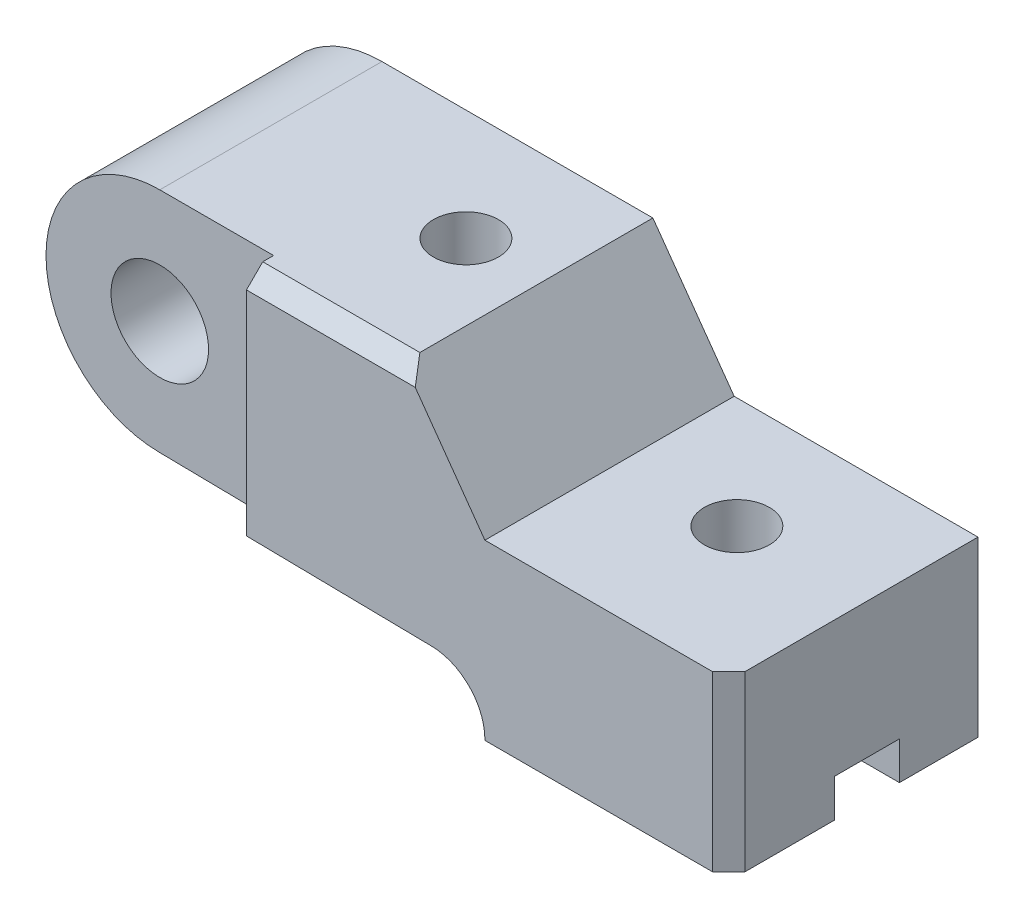
ISO-10303-21;
HEADER;
FILE_DESCRIPTION(('STEP AP214'),'2;1');
FILE_NAME('part.step','',(''),(''),'','','');
FILE_SCHEMA(('AUTOMOTIVE_DESIGN { 1 0 10303 214 1 1 1 1 }'));
ENDSEC;
DATA;
#1=APPLICATION_CONTEXT('core data for automotive mechanical design processes');
#2=APPLICATION_PROTOCOL_DEFINITION('international standard','automotive_design',2000,#1);
#3=PRODUCT_CONTEXT('',#1,'mechanical');
#4=PRODUCT('Part','Part','',(#3));
#5=PRODUCT_RELATED_PRODUCT_CATEGORY('part','',(#4));
#6=PRODUCT_DEFINITION_FORMATION('','',#4);
#7=PRODUCT_DEFINITION_CONTEXT('part definition',#1,'design');
#8=PRODUCT_DEFINITION('design','',#6,#7);
#9=PRODUCT_DEFINITION_SHAPE('','',#8);
#10=(LENGTH_UNIT() NAMED_UNIT(*) SI_UNIT(.MILLI.,.METRE.));
#11=(NAMED_UNIT(*) PLANE_ANGLE_UNIT() SI_UNIT($,.RADIAN.));
#12=(NAMED_UNIT(*) SI_UNIT($,.STERADIAN.) SOLID_ANGLE_UNIT());
#13=UNCERTAINTY_MEASURE_WITH_UNIT(LENGTH_MEASURE(1.E-05),#10,'distance_accuracy_value','');
#14=(GEOMETRIC_REPRESENTATION_CONTEXT(3) GLOBAL_UNCERTAINTY_ASSIGNED_CONTEXT((#13)) GLOBAL_UNIT_ASSIGNED_CONTEXT((#10,
#11,#12)) REPRESENTATION_CONTEXT('',''));
#15=CARTESIAN_POINT('',(0.,0.,0.));
#16=DIRECTION('',(0.,0.,1.));
#17=DIRECTION('',(1.,0.,0.));
#18=AXIS2_PLACEMENT_3D('',#15,#16,#17);
#19=CARTESIAN_POINT('',(0.,-25.,26.5));
#20=DIRECTION('',(0.,1.,0.));
#21=DIRECTION('',(0.,0.,1.));
#22=AXIS2_PLACEMENT_3D('',#19,#20,#21);
#23=PLANE('',#22);
#24=DIRECTION('',(1.,0.,0.));
#25=VECTOR('',#24,1.);
#26=CARTESIAN_POINT('',(0.,-25.,26.5));
#27=LINE('',#26,#25);
#28=CARTESIAN_POINT('',(21.,-25.,26.5));
#29=VERTEX_POINT('',#28);
#30=CARTESIAN_POINT('',(45.,-25.,26.5));
#31=VERTEX_POINT('',#30);
#32=EDGE_CURVE('E339',#29,#31,#27,.T.);
#33=ORIENTED_EDGE('',*,*,#32,.F.);
#34=CARTESIAN_POINT('',(21.,-25.,20.5));
#35=DIRECTION('',(0.,1.,0.));
#36=DIRECTION('',(0.,0.,1.));
#37=AXIS2_PLACEMENT_3D('',#34,#35,#36);
#38=CIRCLE('',#37,6.);
#39=CARTESIAN_POINT('',(21.,-25.,14.5));
#40=VERTEX_POINT('',#39);
#41=EDGE_CURVE('E223',#29,#40,#38,.T.);
#42=ORIENTED_EDGE('',*,*,#41,.T.);
#43=DIRECTION('',(1.,0.,0.));
#44=VECTOR('',#43,1.);
#45=CARTESIAN_POINT('',(0.,-25.,14.5));
#46=LINE('',#45,#44);
#47=CARTESIAN_POINT('',(45.,-25.,14.5));
#48=VERTEX_POINT('',#47);
#49=EDGE_CURVE('E338',#40,#48,#46,.T.);
#50=ORIENTED_EDGE('',*,*,#49,.T.);
#51=DIRECTION('',(0.,0.,1.));
#52=VECTOR('',#51,1.);
#53=CARTESIAN_POINT('',(45.,-25.,26.5));
#54=LINE('',#53,#52);
#55=EDGE_CURVE('E684',#48,#31,#54,.T.);
#56=ORIENTED_EDGE('',*,*,#55,.T.);
#57=EDGE_LOOP('',(#33,#42,#50,#56));
#58=FACE_BOUND('',#57,.T.);
#59=ADVANCED_FACE('F43',(#58),#23,.F.);
#60=CARTESIAN_POINT('',(0.,0.,41.));
#61=DIRECTION('',(1.,0.,0.));
#62=DIRECTION('',(0.,0.,-1.));
#63=AXIS2_PLACEMENT_3D('',#60,#61,#62);
#64=PLANE('',#63);
#65=DIRECTION('',(0.,0.,1.));
#66=VECTOR('',#65,1.);
#67=CARTESIAN_POINT('',(0.,-31.6923440991361,0.));
#68=LINE('',#67,#66);
#69=CARTESIAN_POINT('',(0.,-31.6923440991361,0.));
#70=VERTEX_POINT('',#69);
#71=CARTESIAN_POINT('',(0.,-31.6923440991361,14.5));
#72=VERTEX_POINT('',#71);
#73=EDGE_CURVE('E259',#70,#72,#68,.T.);
#74=ORIENTED_EDGE('',*,*,#73,.F.);
#75=DIRECTION('',(0.,-1.,0.));
#76=VECTOR('',#75,1.);
#77=CARTESIAN_POINT('',(0.,0.,0.));
#78=LINE('',#77,#76);
#79=CARTESIAN_POINT('',(0.,-32.,0.));
#80=VERTEX_POINT('',#79);
#81=EDGE_CURVE('E353',#70,#80,#78,.T.);
#82=ORIENTED_EDGE('',*,*,#81,.T.);
#83=DIRECTION('',(0.,0.,-1.));
#84=VECTOR('',#83,1.);
#85=CARTESIAN_POINT('',(0.,-32.,41.));
#86=LINE('',#85,#84);
#87=CARTESIAN_POINT('',(0.,-32.,14.5));
#88=VERTEX_POINT('',#87);
#89=EDGE_CURVE('E270',#88,#80,#86,.T.);
#90=ORIENTED_EDGE('',*,*,#89,.F.);
#91=DIRECTION('',(0.,1.,0.));
#92=VECTOR('',#91,1.);
#93=CARTESIAN_POINT('',(0.,-25.,14.5));
#94=LINE('',#93,#92);
#95=EDGE_CURVE('E677',#88,#72,#94,.T.);
#96=ORIENTED_EDGE('',*,*,#95,.T.);
#97=EDGE_LOOP('',(#74,#82,#90,#96));
#98=FACE_BOUND('',#97,.T.);
#99=ADVANCED_FACE('F276',(#98),#64,.F.);
#100=CARTESIAN_POINT('',(0.,-31.6923440991361,26.5));
#101=VERTEX_POINT('',#100);
#102=CARTESIAN_POINT('',(0.,-31.6923440991361,41.));
#103=VERTEX_POINT('',#102);
#104=EDGE_CURVE('E262',#101,#103,#68,.T.);
#105=ORIENTED_EDGE('',*,*,#104,.F.);
#106=DIRECTION('',(0.,-1.,0.));
#107=VECTOR('',#106,1.);
#108=CARTESIAN_POINT('',(0.,-32.,26.5));
#109=LINE('',#108,#107);
#110=CARTESIAN_POINT('',(0.,-32.,26.5));
#111=VERTEX_POINT('',#110);
#112=EDGE_CURVE('E685',#101,#111,#109,.T.);
#113=ORIENTED_EDGE('',*,*,#112,.T.);
#114=CARTESIAN_POINT('',(0.,-32.,41.));
#115=VERTEX_POINT('',#114);
#116=EDGE_CURVE('E267',#115,#111,#86,.T.);
#117=ORIENTED_EDGE('',*,*,#116,.F.);
#118=CARTESIAN_POINT('',(-9.99881677808259,-31.846172049568,41.));
#119=DIRECTION('',(0.,0.,-1.));
#120=DIRECTION('',(0.999881677808259,0.0153827950431833,0.));
#121=AXIS2_PLACEMENT_3D('',#118,#119,#120);
#122=CIRCLE('',#121,10.);
#123=EDGE_CURVE('E204',#103,#115,#122,.T.);
#124=ORIENTED_EDGE('',*,*,#123,.F.);
#125=EDGE_LOOP('',(#105,#113,#117,#124));
#126=FACE_BOUND('',#125,.T.);
#127=ADVANCED_FACE('F287',(#126),#64,.F.);
#128=CARTESIAN_POINT('',(45.,-32.,41.));
#129=DIRECTION('',(0.,1.,0.));
#130=DIRECTION('',(0.,0.,1.));
#131=AXIS2_PLACEMENT_3D('',#128,#129,#130);
#132=PLANE('',#131);
#133=DIRECTION('',(0.,0.,-1.));
#134=VECTOR('',#133,1.);
#135=CARTESIAN_POINT('',(45.,-32.,41.));
#136=LINE('',#135,#134);
#137=CARTESIAN_POINT('',(45.,-32.,43.));
#138=VERTEX_POINT('',#137);
#139=CARTESIAN_POINT('',(45.,-32.,26.5));
#140=VERTEX_POINT('',#139);
#141=EDGE_CURVE('E366',#138,#140,#136,.T.);
#142=ORIENTED_EDGE('',*,*,#141,.F.);
#143=DIRECTION('',(-0.707106781186546,0.,0.707106781186549));
#144=VECTOR('',#143,1.);
#145=CARTESIAN_POINT('',(42.,-32.,46.));
#146=LINE('',#145,#144);
#147=CARTESIAN_POINT('',(42.,-32.,46.));
#148=VERTEX_POINT('',#147);
#149=EDGE_CURVE('E11',#138,#148,#146,.T.);
#150=ORIENTED_EDGE('',*,*,#149,.T.);
#151=DIRECTION('',(1.,0.,0.));
#152=VECTOR('',#151,1.);
#153=CARTESIAN_POINT('',(0.,-32.,46.));
#154=LINE('',#153,#152);
#155=CARTESIAN_POINT('',(0.,-32.,46.));
#156=VERTEX_POINT('',#155);
#157=EDGE_CURVE('E176',#156,#148,#154,.T.);
#158=ORIENTED_EDGE('',*,*,#157,.F.);
#159=DIRECTION('',(0.,0.,-1.));
#160=VECTOR('',#159,1.);
#161=CARTESIAN_POINT('',(0.,-32.,46.));
#162=LINE('',#161,#160);
#163=EDGE_CURVE('E181',#156,#115,#162,.T.);
#164=ORIENTED_EDGE('',*,*,#163,.T.);
#165=ORIENTED_EDGE('',*,*,#116,.T.);
#166=DIRECTION('',(1.,0.,0.));
#167=VECTOR('',#166,1.);
#168=CARTESIAN_POINT('',(0.,-32.,26.5));
#169=LINE('',#168,#167);
#170=EDGE_CURVE('E350',#111,#140,#169,.T.);
#171=ORIENTED_EDGE('',*,*,#170,.T.);
#172=EDGE_LOOP('',(#142,#150,#158,#164,#165,#171));
#173=FACE_BOUND('',#172,.T.);
#174=ADVANCED_FACE('F178',(#173),#132,.F.);
#175=CARTESIAN_POINT('',(45.,-32.,14.5));
#176=VERTEX_POINT('',#175);
#177=CARTESIAN_POINT('',(45.,-32.,0.));
#178=VERTEX_POINT('',#177);
#179=EDGE_CURVE('E362',#176,#178,#136,.T.);
#180=ORIENTED_EDGE('',*,*,#179,.F.);
#181=DIRECTION('',(1.,0.,0.));
#182=VECTOR('',#181,1.);
#183=CARTESIAN_POINT('',(0.,-32.,14.5));
#184=LINE('',#183,#182);
#185=EDGE_CURVE('E341',#88,#176,#184,.T.);
#186=ORIENTED_EDGE('',*,*,#185,.F.);
#187=ORIENTED_EDGE('',*,*,#89,.T.);
#188=DIRECTION('',(1.,0.,0.));
#189=VECTOR('',#188,1.);
#190=CARTESIAN_POINT('',(45.,-32.,0.));
#191=LINE('',#190,#189);
#192=EDGE_CURVE('E352',#80,#178,#191,.T.);
#193=ORIENTED_EDGE('',*,*,#192,.T.);
#194=EDGE_LOOP('',(#180,#186,#187,#193));
#195=FACE_BOUND('',#194,.T.);
#196=ADVANCED_FACE('F286',(#195),#132,.F.);
#197=CARTESIAN_POINT('',(45.,0.,41.));
#198=DIRECTION('',(-1.,0.,0.));
#199=DIRECTION('',(0.,0.,1.));
#200=AXIS2_PLACEMENT_3D('',#197,#198,#199);
#201=PLANE('',#200);
#202=DIRECTION('',(0.,0.,-1.));
#203=VECTOR('',#202,1.);
#204=CARTESIAN_POINT('',(45.,0.,41.));
#205=LINE('',#204,#203);
#206=CARTESIAN_POINT('',(45.,0.,43.));
#207=VERTEX_POINT('',#206);
#208=CARTESIAN_POINT('',(45.,0.,0.));
#209=VERTEX_POINT('',#208);
#210=EDGE_CURVE('E364',#207,#209,#205,.T.);
#211=ORIENTED_EDGE('',*,*,#210,.F.);
#212=DIRECTION('',(0.,-1.,0.));
#213=VECTOR('',#212,1.);
#214=CARTESIAN_POINT('',(45.,-32.,43.));
#215=LINE('',#214,#213);
#216=EDGE_CURVE('E55',#207,#138,#215,.T.);
#217=ORIENTED_EDGE('',*,*,#216,.T.);
#218=ORIENTED_EDGE('',*,*,#141,.T.);
#219=DIRECTION('',(0.,-1.,0.));
#220=VECTOR('',#219,1.);
#221=CARTESIAN_POINT('',(45.,-32.,26.5));
#222=LINE('',#221,#220);
#223=EDGE_CURVE('E249',#31,#140,#222,.T.);
#224=ORIENTED_EDGE('',*,*,#223,.F.);
#225=ORIENTED_EDGE('',*,*,#55,.F.);
#226=DIRECTION('',(0.,1.,0.));
#227=VECTOR('',#226,1.);
#228=CARTESIAN_POINT('',(45.,-25.,14.5));
#229=LINE('',#228,#227);
#230=EDGE_CURVE('E380',#176,#48,#229,.T.);
#231=ORIENTED_EDGE('',*,*,#230,.F.);
#232=ORIENTED_EDGE('',*,*,#179,.T.);
#233=DIRECTION('',(0.,1.,0.));
#234=VECTOR('',#233,1.);
#235=CARTESIAN_POINT('',(45.,0.,0.));
#236=LINE('',#235,#234);
#237=EDGE_CURVE('E358',#178,#209,#236,.T.);
#238=ORIENTED_EDGE('',*,*,#237,.T.);
#239=EDGE_LOOP('',(#211,#217,#218,#224,#225,#231,#232,#238));
#240=FACE_BOUND('',#239,.T.);
#241=ADVANCED_FACE('F375',(#240),#201,.F.);
#242=CARTESIAN_POINT('',(0.,0.,41.));
#243=DIRECTION('',(0.,-1.,0.));
#244=DIRECTION('',(0.,0.,-1.));
#245=AXIS2_PLACEMENT_3D('',#242,#243,#244);
#246=PLANE('',#245);
#247=CARTESIAN_POINT('',(21.,0.,20.5));
#248=DIRECTION('',(0.,-1.,0.));
#249=DIRECTION('',(0.,0.,-1.));
#250=AXIS2_PLACEMENT_3D('',#247,#248,#249);
#251=CIRCLE('',#250,6.);
#252=CARTESIAN_POINT('',(21.,0.,14.5));
#253=VERTEX_POINT('',#252);
#254=EDGE_CURVE('E224',#253,#253,#251,.T.);
#255=ORIENTED_EDGE('',*,*,#254,.T.);
#256=EDGE_LOOP('',(#255));
#257=FACE_BOUND('',#256,.T.);
#258=DIRECTION('',(-1.,0.,0.));
#259=VECTOR('',#258,1.);
#260=CARTESIAN_POINT('',(0.,0.,46.));
#261=LINE('',#260,#259);
#262=CARTESIAN_POINT('',(42.,0.,46.));
#263=VERTEX_POINT('',#262);
#264=CARTESIAN_POINT('',(0.,0.,46.));
#265=VERTEX_POINT('',#264);
#266=EDGE_CURVE('E190',#263,#265,#261,.T.);
#267=ORIENTED_EDGE('',*,*,#266,.F.);
#268=DIRECTION('',(0.707106781186546,0.,-0.707106781186549));
#269=VECTOR('',#268,1.);
#270=CARTESIAN_POINT('',(42.,0.,46.));
#271=LINE('',#270,#269);
#272=EDGE_CURVE('E69',#263,#207,#271,.T.);
#273=ORIENTED_EDGE('',*,*,#272,.T.);
#274=ORIENTED_EDGE('',*,*,#210,.T.);
#275=DIRECTION('',(-1.,0.,0.));
#276=VECTOR('',#275,1.);
#277=CARTESIAN_POINT('',(0.,0.,0.));
#278=LINE('',#277,#276);
#279=CARTESIAN_POINT('',(0.,0.,0.));
#280=VERTEX_POINT('',#279);
#281=EDGE_CURVE('E360',#209,#280,#278,.T.);
#282=ORIENTED_EDGE('',*,*,#281,.T.);
#283=DIRECTION('',(0.,0.,-1.));
#284=VECTOR('',#283,1.);
#285=CARTESIAN_POINT('',(0.,0.,41.));
#286=LINE('',#285,#284);
#287=EDGE_CURVE('E363',#265,#280,#286,.T.);
#288=ORIENTED_EDGE('',*,*,#287,.F.);
#289=EDGE_LOOP('',(#267,#273,#274,#282,#288));
#290=FACE_BOUND('',#289,.T.);
#291=ADVANCED_FACE('F387',(#257,#290),#246,.F.);
#292=CARTESIAN_POINT('',(0.,0.,41.));
#293=DIRECTION('',(0.,0.,-1.));
#294=DIRECTION('',(-1.,0.,0.));
#295=AXIS2_PLACEMENT_3D('',#292,#293,#294);
#296=PLANE('',#295);
#297=CARTESIAN_POINT('',(-65.,8.11850586757146E-13,41.));
#298=DIRECTION('',(0.,0.,1.));
#299=DIRECTION('',(1.,0.,0.));
#300=AXIS2_PLACEMENT_3D('',#297,#298,#299);
#301=CIRCLE('',#300,9.);
#302=CARTESIAN_POINT('',(-56.,8.11850586757146E-13,41.));
#303=VERTEX_POINT('',#302);
#304=EDGE_CURVE('E401',#303,#303,#301,.T.);
#305=ORIENTED_EDGE('',*,*,#304,.F.);
#306=EDGE_LOOP('',(#305));
#307=FACE_BOUND('',#306,.T.);
#308=DIRECTION('',(0.999881677808259,-0.0153827950432186,0.));
#309=VECTOR('',#308,1.);
#310=CARTESIAN_POINT('',(-0.33838144817827,-21.9947941315666,41.));
#311=LINE('',#310,#309);
#312=CARTESIAN_POINT('',(-65.,-20.9999999999992,41.));
#313=VERTEX_POINT('',#312);
#314=CARTESIAN_POINT('',(-44.,-21.3230769230764,41.));
#315=VERTEX_POINT('',#314);
#316=EDGE_CURVE('E230',#313,#315,#311,.T.);
#317=ORIENTED_EDGE('',*,*,#316,.T.);
#318=DIRECTION('',(0.,1.,0.));
#319=VECTOR('',#318,1.);
#320=CARTESIAN_POINT('',(-44.,0.,41.));
#321=LINE('',#320,#319);
#322=CARTESIAN_POINT('',(-44.,21.0000000000008,41.));
#323=VERTEX_POINT('',#322);
#324=EDGE_CURVE('E200',#315,#323,#321,.T.);
#325=ORIENTED_EDGE('',*,*,#324,.T.);
#326=DIRECTION('',(1.,0.,0.));
#327=VECTOR('',#326,1.);
#328=CARTESIAN_POINT('',(0.,21.0000000000008,41.));
#329=LINE('',#328,#327);
#330=CARTESIAN_POINT('',(-65.,21.0000000000008,41.));
#331=VERTEX_POINT('',#330);
#332=EDGE_CURVE('E221',#331,#323,#329,.T.);
#333=ORIENTED_EDGE('',*,*,#332,.F.);
#334=CARTESIAN_POINT('',(-65.,8.11850586757146E-13,41.));
#335=DIRECTION('',(0.,0.,1.));
#336=DIRECTION('',(1.,0.,0.));
#337=AXIS2_PLACEMENT_3D('',#334,#335,#336);
#338=CIRCLE('',#337,21.);
#339=EDGE_CURVE('E243',#331,#313,#338,.T.);
#340=ORIENTED_EDGE('',*,*,#339,.T.);
#341=EDGE_LOOP('',(#317,#325,#333,#340));
#342=FACE_BOUND('',#341,.T.);
#343=ADVANCED_FACE('F582',(#307,#342),#296,.F.);
#344=CARTESIAN_POINT('',(0.,0.,0.));
#345=DIRECTION('',(0.,0.,-1.));
#346=DIRECTION('',(-1.,0.,0.));
#347=AXIS2_PLACEMENT_3D('',#344,#345,#346);
#348=PLANE('',#347);
#349=CARTESIAN_POINT('',(-65.,8.11850586757146E-13,0.));
#350=DIRECTION('',(0.,0.,-1.));
#351=DIRECTION('',(-1.,0.,0.));
#352=AXIS2_PLACEMENT_3D('',#349,#350,#351);
#353=CIRCLE('',#352,9.);
#354=CARTESIAN_POINT('',(-74.,8.11850586757146E-13,0.));
#355=VERTEX_POINT('',#354);
#356=EDGE_CURVE('E402',#355,#355,#353,.T.);
#357=ORIENTED_EDGE('',*,*,#356,.F.);
#358=EDGE_LOOP('',(#357));
#359=FACE_BOUND('',#358,.T.);
#360=ORIENTED_EDGE('',*,*,#81,.F.);
#361=CARTESIAN_POINT('',(-9.99881677808259,-31.846172049568,0.));
#362=DIRECTION('',(0.,0.,1.));
#363=DIRECTION('',(1.,0.,0.));
#364=AXIS2_PLACEMENT_3D('',#361,#362,#363);
#365=CIRCLE('',#364,10.);
#366=CARTESIAN_POINT('',(-9.9988167780826,-21.846172049568,0.));
#367=VERTEX_POINT('',#366);
#368=EDGE_CURVE('E228',#70,#367,#365,.T.);
#369=ORIENTED_EDGE('',*,*,#368,.T.);
#370=DIRECTION('',(0.999881677808259,-0.0153827950432186,0.));
#371=VECTOR('',#370,1.);
#372=CARTESIAN_POINT('',(-0.33838144817827,-21.9947941315666,0.));
#373=LINE('',#372,#371);
#374=CARTESIAN_POINT('',(-65.,-20.9999999999992,0.));
#375=VERTEX_POINT('',#374);
#376=EDGE_CURVE('E240',#375,#367,#373,.T.);
#377=ORIENTED_EDGE('',*,*,#376,.F.);
#378=CARTESIAN_POINT('',(-65.,8.11850586757146E-13,0.));
#379=DIRECTION('',(0.,0.,1.));
#380=DIRECTION('',(1.,0.,0.));
#381=AXIS2_PLACEMENT_3D('',#378,#379,#380);
#382=CIRCLE('',#381,21.);
#383=CARTESIAN_POINT('',(-65.,21.0000000000008,0.));
#384=VERTEX_POINT('',#383);
#385=EDGE_CURVE('E234',#384,#375,#382,.T.);
#386=ORIENTED_EDGE('',*,*,#385,.F.);
#387=DIRECTION('',(1.,0.,0.));
#388=VECTOR('',#387,1.);
#389=CARTESIAN_POINT('',(0.,21.0000000000008,0.));
#390=LINE('',#389,#388);
#391=CARTESIAN_POINT('',(-15.,21.0000000000008,0.));
#392=VERTEX_POINT('',#391);
#393=EDGE_CURVE('E235',#384,#392,#390,.T.);
#394=ORIENTED_EDGE('',*,*,#393,.T.);
#395=DIRECTION('',(0.581238193719081,-0.813733471206746,0.));
#396=VECTOR('',#395,1.);
#397=CARTESIAN_POINT('',(0.,0.,0.));
#398=LINE('',#397,#396);
#399=EDGE_CURVE('E226',#392,#280,#398,.T.);
#400=ORIENTED_EDGE('',*,*,#399,.T.);
#401=ORIENTED_EDGE('',*,*,#281,.F.);
#402=ORIENTED_EDGE('',*,*,#237,.F.);
#403=ORIENTED_EDGE('',*,*,#192,.F.);
#404=EDGE_LOOP('',(#360,#369,#377,#386,#394,#400,#401,#402,#403));
#405=FACE_BOUND('',#404,.T.);
#406=ADVANCED_FACE('F328',(#359,#405),#348,.T.);
#407=CARTESIAN_POINT('',(0.,-32.,26.5));
#408=DIRECTION('',(0.,0.,1.));
#409=DIRECTION('',(1.,0.,0.));
#410=AXIS2_PLACEMENT_3D('',#407,#408,#409);
#411=PLANE('',#410);
#412=CARTESIAN_POINT('',(0.,-25.,26.5));
#413=VERTEX_POINT('',#412);
#414=EDGE_CURVE('E345',#413,#29,#27,.T.);
#415=ORIENTED_EDGE('',*,*,#414,.T.);
#416=ORIENTED_EDGE('',*,*,#32,.T.);
#417=ORIENTED_EDGE('',*,*,#223,.T.);
#418=ORIENTED_EDGE('',*,*,#170,.F.);
#419=ORIENTED_EDGE('',*,*,#112,.F.);
#420=EDGE_CURVE('E261',#413,#101,#109,.T.);
#421=ORIENTED_EDGE('',*,*,#420,.F.);
#422=EDGE_LOOP('',(#415,#416,#417,#418,#419,#421));
#423=FACE_BOUND('',#422,.T.);
#424=ADVANCED_FACE('F325',(#423),#411,.F.);
#425=CARTESIAN_POINT('',(0.,-25.,14.5));
#426=VERTEX_POINT('',#425);
#427=EDGE_CURVE('E335',#426,#40,#46,.T.);
#428=ORIENTED_EDGE('',*,*,#427,.T.);
#429=EDGE_CURVE('E220',#40,#29,#38,.T.);
#430=ORIENTED_EDGE('',*,*,#429,.T.);
#431=ORIENTED_EDGE('',*,*,#414,.F.);
#432=DIRECTION('',(0.,0.,1.));
#433=VECTOR('',#432,1.);
#434=CARTESIAN_POINT('',(0.,-25.,26.5));
#435=LINE('',#434,#433);
#436=EDGE_CURVE('E337',#426,#413,#435,.T.);
#437=ORIENTED_EDGE('',*,*,#436,.F.);
#438=EDGE_LOOP('',(#428,#430,#431,#437));
#439=FACE_BOUND('',#438,.T.);
#440=ADVANCED_FACE('F315',(#439),#23,.F.);
#441=CARTESIAN_POINT('',(0.,-25.,14.5));
#442=DIRECTION('',(0.,0.,-1.));
#443=DIRECTION('',(-1.,0.,0.));
#444=AXIS2_PLACEMENT_3D('',#441,#442,#443);
#445=PLANE('',#444);
#446=ORIENTED_EDGE('',*,*,#49,.F.);
#447=ORIENTED_EDGE('',*,*,#427,.F.);
#448=EDGE_CURVE('E680',#72,#426,#94,.T.);
#449=ORIENTED_EDGE('',*,*,#448,.F.);
#450=ORIENTED_EDGE('',*,*,#95,.F.);
#451=ORIENTED_EDGE('',*,*,#185,.T.);
#452=ORIENTED_EDGE('',*,*,#230,.T.);
#453=EDGE_LOOP('',(#446,#447,#449,#450,#451,#452));
#454=FACE_BOUND('',#453,.T.);
#455=ADVANCED_FACE('F322',(#454),#445,.F.);
#456=CARTESIAN_POINT('',(0.,0.,0.));
#457=DIRECTION('',(-1.,0.,0.));
#458=DIRECTION('',(0.,0.,1.));
#459=AXIS2_PLACEMENT_3D('',#456,#457,#458);
#460=PLANE('',#459);
#461=ORIENTED_EDGE('',*,*,#436,.T.);
#462=ORIENTED_EDGE('',*,*,#420,.T.);
#463=EDGE_CURVE('E239',#72,#101,#68,.T.);
#464=ORIENTED_EDGE('',*,*,#463,.F.);
#465=ORIENTED_EDGE('',*,*,#448,.T.);
#466=EDGE_LOOP('',(#461,#462,#464,#465));
#467=FACE_BOUND('',#466,.T.);
#468=ADVANCED_FACE('F326',(#467),#460,.F.);
#469=CARTESIAN_POINT('',(-9.99881677808259,-31.846172049568,0.));
#470=DIRECTION('',(0.,0.,1.));
#471=DIRECTION('',(1.,0.,0.));
#472=AXIS2_PLACEMENT_3D('',#469,#470,#471);
#473=CYLINDRICAL_SURFACE('',#472,10.);
#474=ORIENTED_EDGE('',*,*,#104,.T.);
#475=ORIENTED_EDGE('',*,*,#123,.T.);
#476=ORIENTED_EDGE('',*,*,#163,.F.);
#477=CARTESIAN_POINT('',(-9.99881677808259,-31.846172049568,46.));
#478=DIRECTION('',(0.,0.,1.));
#479=DIRECTION('',(1.,0.,0.));
#480=AXIS2_PLACEMENT_3D('',#477,#478,#479);
#481=CIRCLE('',#480,10.);
#482=CARTESIAN_POINT('',(-9.9988167780826,-21.846172049568,46.));
#483=VERTEX_POINT('',#482);
#484=EDGE_CURVE('E189',#483,#156,#481,.F.);
#485=ORIENTED_EDGE('',*,*,#484,.F.);
#486=DIRECTION('',(0.,0.,1.));
#487=VECTOR('',#486,1.);
#488=CARTESIAN_POINT('',(-9.9988167780826,-21.846172049568,0.));
#489=LINE('',#488,#487);
#490=EDGE_CURVE('E247',#367,#483,#489,.T.);
#491=ORIENTED_EDGE('',*,*,#490,.F.);
#492=ORIENTED_EDGE('',*,*,#368,.F.);
#493=ORIENTED_EDGE('',*,*,#73,.T.);
#494=ORIENTED_EDGE('',*,*,#463,.T.);
#495=EDGE_LOOP('',(#474,#475,#476,#485,#491,#492,#493,#494));
#496=FACE_BOUND('',#495,.T.);
#497=ADVANCED_FACE('F203',(#496),#473,.F.);
#498=CARTESIAN_POINT('',(-0.33838144817827,-21.9947941315666,0.));
#499=DIRECTION('',(-0.0153827950432186,-0.999881677808259,0.));
#500=DIRECTION('',(0.999881677808259,-0.0153827950432186,0.));
#501=AXIS2_PLACEMENT_3D('',#498,#499,#500);
#502=PLANE('',#501);
#503=CARTESIAN_POINT('',(-29.,-21.5538461538459,20.5));
#504=DIRECTION('',(-0.0153827950432186,-0.999881677808259,0.));
#505=DIRECTION('',(-0.999881677808259,0.0153827950432186,0.));
#506=AXIS2_PLACEMENT_3D('',#503,#504,#505);
#507=ELLIPSE('',#506,6.00071001716124,6.);
#508=CARTESIAN_POINT('',(-35.,-21.4615384615381,20.5));
#509=VERTEX_POINT('',#508);
#510=EDGE_CURVE('E206',#509,#509,#507,.T.);
#511=ORIENTED_EDGE('',*,*,#510,.F.);
#512=EDGE_LOOP('',(#511));
#513=FACE_BOUND('',#512,.T.);
#514=ORIENTED_EDGE('',*,*,#316,.F.);
#515=DIRECTION('',(0.,0.,1.));
#516=VECTOR('',#515,1.);
#517=CARTESIAN_POINT('',(-65.,-20.9999999999992,0.));
#518=LINE('',#517,#516);
#519=EDGE_CURVE('E252',#375,#313,#518,.T.);
#520=ORIENTED_EDGE('',*,*,#519,.F.);
#521=ORIENTED_EDGE('',*,*,#376,.T.);
#522=ORIENTED_EDGE('',*,*,#490,.T.);
#523=DIRECTION('',(0.999881677808259,-0.0153827950432186,0.));
#524=VECTOR('',#523,1.);
#525=CARTESIAN_POINT('',(-0.33838144817827,-21.9947941315666,46.));
#526=LINE('',#525,#524);
#527=CARTESIAN_POINT('',(-44.,-21.3230769230764,46.));
#528=VERTEX_POINT('',#527);
#529=EDGE_CURVE('E193',#528,#483,#526,.T.);
#530=ORIENTED_EDGE('',*,*,#529,.F.);
#531=DIRECTION('',(0.,0.,-1.));
#532=VECTOR('',#531,1.);
#533=CARTESIAN_POINT('',(-44.,-21.3230769230764,46.));
#534=LINE('',#533,#532);
#535=EDGE_CURVE('E208',#528,#315,#534,.T.);
#536=ORIENTED_EDGE('',*,*,#535,.T.);
#537=EDGE_LOOP('',(#514,#520,#521,#522,#530,#536));
#538=FACE_BOUND('',#537,.T.);
#539=ADVANCED_FACE('F413',(#513,#538),#502,.T.);
#540=CARTESIAN_POINT('',(-65.,8.11850586757146E-13,0.));
#541=DIRECTION('',(0.,0.,1.));
#542=DIRECTION('',(1.,0.,0.));
#543=AXIS2_PLACEMENT_3D('',#540,#541,#542);
#544=CYLINDRICAL_SURFACE('',#543,21.);
#545=ORIENTED_EDGE('',*,*,#339,.F.);
#546=DIRECTION('',(0.,0.,1.));
#547=VECTOR('',#546,1.);
#548=CARTESIAN_POINT('',(-65.,21.0000000000008,0.));
#549=LINE('',#548,#547);
#550=EDGE_CURVE('E254',#384,#331,#549,.T.);
#551=ORIENTED_EDGE('',*,*,#550,.F.);
#552=ORIENTED_EDGE('',*,*,#385,.T.);
#553=ORIENTED_EDGE('',*,*,#519,.T.);
#554=EDGE_LOOP('',(#545,#551,#552,#553));
#555=FACE_BOUND('',#554,.T.);
#556=ADVANCED_FACE('F428',(#555),#544,.T.);
#557=CARTESIAN_POINT('',(0.,21.0000000000008,0.));
#558=DIRECTION('',(0.,-1.,0.));
#559=DIRECTION('',(0.,0.,-1.));
#560=AXIS2_PLACEMENT_3D('',#557,#558,#559);
#561=PLANE('',#560);
#562=CARTESIAN_POINT('',(-29.,21.0000000000008,20.5));
#563=DIRECTION('',(0.,1.,0.));
#564=DIRECTION('',(0.,0.,1.));
#565=AXIS2_PLACEMENT_3D('',#562,#563,#564);
#566=CIRCLE('',#565,6.);
#567=CARTESIAN_POINT('',(-29.,21.0000000000008,26.5));
#568=VERTEX_POINT('',#567);
#569=EDGE_CURVE('E205',#568,#568,#566,.T.);
#570=ORIENTED_EDGE('',*,*,#569,.F.);
#571=EDGE_LOOP('',(#570));
#572=FACE_BOUND('',#571,.T.);
#573=DIRECTION('',(0.,0.,-1.));
#574=VECTOR('',#573,1.);
#575=CARTESIAN_POINT('',(-44.,21.0000000000008,46.));
#576=LINE('',#575,#574);
#577=CARTESIAN_POINT('',(-44.,21.0000000000008,43.));
#578=VERTEX_POINT('',#577);
#579=EDGE_CURVE('E201',#578,#323,#576,.T.);
#580=ORIENTED_EDGE('',*,*,#579,.F.);
#581=DIRECTION('',(1.,0.,0.));
#582=VECTOR('',#581,1.);
#583=CARTESIAN_POINT('',(-15.,21.0000000000008,43.));
#584=LINE('',#583,#582);
#585=CARTESIAN_POINT('',(-15.,21.0000000000008,43.));
#586=VERTEX_POINT('',#585);
#587=EDGE_CURVE('E393',#578,#586,#584,.T.);
#588=ORIENTED_EDGE('',*,*,#587,.T.);
#589=DIRECTION('',(0.,0.,1.));
#590=VECTOR('',#589,1.);
#591=CARTESIAN_POINT('',(-15.,21.0000000000008,0.));
#592=LINE('',#591,#590);
#593=EDGE_CURVE('E253',#392,#586,#592,.T.);
#594=ORIENTED_EDGE('',*,*,#593,.F.);
#595=ORIENTED_EDGE('',*,*,#393,.F.);
#596=ORIENTED_EDGE('',*,*,#550,.T.);
#597=ORIENTED_EDGE('',*,*,#332,.T.);
#598=EDGE_LOOP('',(#580,#588,#594,#595,#596,#597));
#599=FACE_BOUND('',#598,.T.);
#600=ADVANCED_FACE('F422',(#572,#599),#561,.F.);
#601=CARTESIAN_POINT('',(0.,0.,0.));
#602=DIRECTION('',(-0.813733471206746,-0.581238193719081,0.));
#603=DIRECTION('',(0.581238193719081,-0.813733471206746,0.));
#604=AXIS2_PLACEMENT_3D('',#601,#602,#603);
#605=PLANE('',#604);
#606=ORIENTED_EDGE('',*,*,#593,.T.);
#607=DIRECTION('',(0.450834817333701,-0.631168744267206,0.631168744267209));
#608=VECTOR('',#607,1.);
#609=CARTESIAN_POINT('',(-10.2439024390246,14.341463414635,49.6585365853658));
#610=LINE('',#609,#608);
#611=CARTESIAN_POINT('',(-12.8571428571429,18.0000000000008,46.));
#612=VERTEX_POINT('',#611);
#613=EDGE_CURVE('E391',#586,#612,#610,.T.);
#614=ORIENTED_EDGE('',*,*,#613,.T.);
#615=DIRECTION('',(-0.581238193719081,0.813733471206746,0.));
#616=VECTOR('',#615,1.);
#617=CARTESIAN_POINT('',(0.,0.,46.));
#618=LINE('',#617,#616);
#619=EDGE_CURVE('E665',#265,#612,#618,.T.);
#620=ORIENTED_EDGE('',*,*,#619,.F.);
#621=ORIENTED_EDGE('',*,*,#287,.T.);
#622=ORIENTED_EDGE('',*,*,#399,.F.);
#623=EDGE_LOOP('',(#606,#614,#620,#621,#622));
#624=FACE_BOUND('',#623,.T.);
#625=ADVANCED_FACE('F417',(#624),#605,.F.);
#626=CARTESIAN_POINT('',(-29.,-28.9999999999992,20.5));
#627=DIRECTION('',(0.,1.,0.));
#628=DIRECTION('',(0.,0.,1.));
#629=AXIS2_PLACEMENT_3D('',#626,#627,#628);
#630=CYLINDRICAL_SURFACE('',#629,6.);
#631=ORIENTED_EDGE('',*,*,#510,.T.);
#632=EDGE_LOOP('',(#631));
#633=FACE_BOUND('',#632,.T.);
#634=ORIENTED_EDGE('',*,*,#569,.T.);
#635=EDGE_LOOP('',(#634));
#636=FACE_BOUND('',#635,.T.);
#637=ADVANCED_FACE('F423',(#633,#636),#630,.F.);
#638=CARTESIAN_POINT('',(21.,-28.9999999999992,20.5));
#639=DIRECTION('',(0.,1.,0.));
#640=DIRECTION('',(0.,0.,1.));
#641=AXIS2_PLACEMENT_3D('',#638,#639,#640);
#642=CYLINDRICAL_SURFACE('',#641,6.);
#643=ORIENTED_EDGE('',*,*,#429,.F.);
#644=ORIENTED_EDGE('',*,*,#41,.F.);
#645=EDGE_LOOP('',(#643,#644));
#646=FACE_BOUND('',#645,.T.);
#647=ORIENTED_EDGE('',*,*,#254,.F.);
#648=EDGE_LOOP('',(#647));
#649=FACE_BOUND('',#648,.T.);
#650=ADVANCED_FACE('F433',(#646,#649),#642,.F.);
#651=CARTESIAN_POINT('',(-44.,0.,46.));
#652=DIRECTION('',(-1.,0.,0.));
#653=DIRECTION('',(0.,0.,1.));
#654=AXIS2_PLACEMENT_3D('',#651,#652,#653);
#655=PLANE('',#654);
#656=DIRECTION('',(0.,1.,0.));
#657=VECTOR('',#656,1.);
#658=CARTESIAN_POINT('',(-44.,0.,46.));
#659=LINE('',#658,#657);
#660=CARTESIAN_POINT('',(-44.,18.0000000000008,46.));
#661=VERTEX_POINT('',#660);
#662=EDGE_CURVE('E656',#528,#661,#659,.T.);
#663=ORIENTED_EDGE('',*,*,#662,.T.);
#664=DIRECTION('',(0.,0.707106781186546,-0.707106781186549));
#665=VECTOR('',#664,1.);
#666=CARTESIAN_POINT('',(-44.,9.00000000000045,55.0000000000004));
#667=LINE('',#666,#665);
#668=EDGE_CURVE('E398',#661,#578,#667,.T.);
#669=ORIENTED_EDGE('',*,*,#668,.T.);
#670=ORIENTED_EDGE('',*,*,#579,.T.);
#671=ORIENTED_EDGE('',*,*,#324,.F.);
#672=ORIENTED_EDGE('',*,*,#535,.F.);
#673=EDGE_LOOP('',(#663,#669,#670,#671,#672));
#674=FACE_BOUND('',#673,.T.);
#675=ADVANCED_FACE('F436',(#674),#655,.T.);
#676=CARTESIAN_POINT('',(0.,0.,46.));
#677=DIRECTION('',(0.,0.,1.));
#678=DIRECTION('',(1.,0.,0.));
#679=AXIS2_PLACEMENT_3D('',#676,#677,#678);
#680=PLANE('',#679);
#681=ORIENTED_EDGE('',*,*,#157,.T.);
#682=DIRECTION('',(0.,1.,0.));
#683=VECTOR('',#682,1.);
#684=CARTESIAN_POINT('',(42.,0.,46.));
#685=LINE('',#684,#683);
#686=EDGE_CURVE('E389',#148,#263,#685,.T.);
#687=ORIENTED_EDGE('',*,*,#686,.T.);
#688=ORIENTED_EDGE('',*,*,#266,.T.);
#689=ORIENTED_EDGE('',*,*,#619,.T.);
#690=DIRECTION('',(-1.,0.,0.));
#691=VECTOR('',#690,1.);
#692=CARTESIAN_POINT('',(-44.,18.0000000000008,46.));
#693=LINE('',#692,#691);
#694=EDGE_CURVE('E397',#612,#661,#693,.T.);
#695=ORIENTED_EDGE('',*,*,#694,.T.);
#696=ORIENTED_EDGE('',*,*,#662,.F.);
#697=ORIENTED_EDGE('',*,*,#529,.T.);
#698=ORIENTED_EDGE('',*,*,#484,.T.);
#699=EDGE_LOOP('',(#681,#687,#688,#689,#695,#696,#697,#698));
#700=FACE_BOUND('',#699,.T.);
#701=ADVANCED_FACE('F195',(#700),#680,.T.);
#702=CARTESIAN_POINT('',(-65.,8.11850586757146E-13,-9.));
#703=DIRECTION('',(0.,0.,1.));
#704=DIRECTION('',(1.,0.,0.));
#705=AXIS2_PLACEMENT_3D('',#702,#703,#704);
#706=CYLINDRICAL_SURFACE('',#705,9.);
#707=ORIENTED_EDGE('',*,*,#356,.T.);
#708=EDGE_LOOP('',(#707));
#709=FACE_BOUND('',#708,.T.);
#710=ORIENTED_EDGE('',*,*,#304,.T.);
#711=EDGE_LOOP('',(#710));
#712=FACE_BOUND('',#711,.T.);
#713=ADVANCED_FACE('F300',(#709,#712),#706,.F.);
#714=CARTESIAN_POINT('',(0.,18.0000000000008,46.));
#715=DIRECTION('',(0.,0.707106781186549,0.707106781186546));
#716=DIRECTION('',(1.,0.,0.));
#717=AXIS2_PLACEMENT_3D('',#714,#715,#716);
#718=PLANE('',#717);
#719=ORIENTED_EDGE('',*,*,#613,.F.);
#720=ORIENTED_EDGE('',*,*,#587,.F.);
#721=ORIENTED_EDGE('',*,*,#668,.F.);
#722=ORIENTED_EDGE('',*,*,#694,.F.);
#723=EDGE_LOOP('',(#719,#720,#721,#722));
#724=FACE_BOUND('',#723,.T.);
#725=ADVANCED_FACE('F291',(#724),#718,.T.);
#726=CARTESIAN_POINT('',(42.,0.,46.));
#727=DIRECTION('',(0.707106781186549,0.,0.707106781186546));
#728=DIRECTION('',(0.,-1.,0.));
#729=AXIS2_PLACEMENT_3D('',#726,#727,#728);
#730=PLANE('',#729);
#731=ORIENTED_EDGE('',*,*,#149,.F.);
#732=ORIENTED_EDGE('',*,*,#216,.F.);
#733=ORIENTED_EDGE('',*,*,#272,.F.);
#734=ORIENTED_EDGE('',*,*,#686,.F.);
#735=EDGE_LOOP('',(#731,#732,#733,#734));
#736=FACE_BOUND('',#735,.T.);
#737=ADVANCED_FACE('F46',(#736),#730,.T.);
#738=CLOSED_SHELL('',(#59,#99,#127,#174,#196,#241,#291,#343,#406,#424,#440,#455,#468,#497,#539,
#556,#600,#625,#637,#650,#675,#701,#713,#725,#737));
#739=MANIFOLD_SOLID_BREP('B2',#738);
#740=ADVANCED_BREP_SHAPE_REPRESENTATION('',(#18,#739),#14);
#741=SHAPE_DEFINITION_REPRESENTATION(#9,#740);
ENDSEC;
END-ISO-10303-21;
